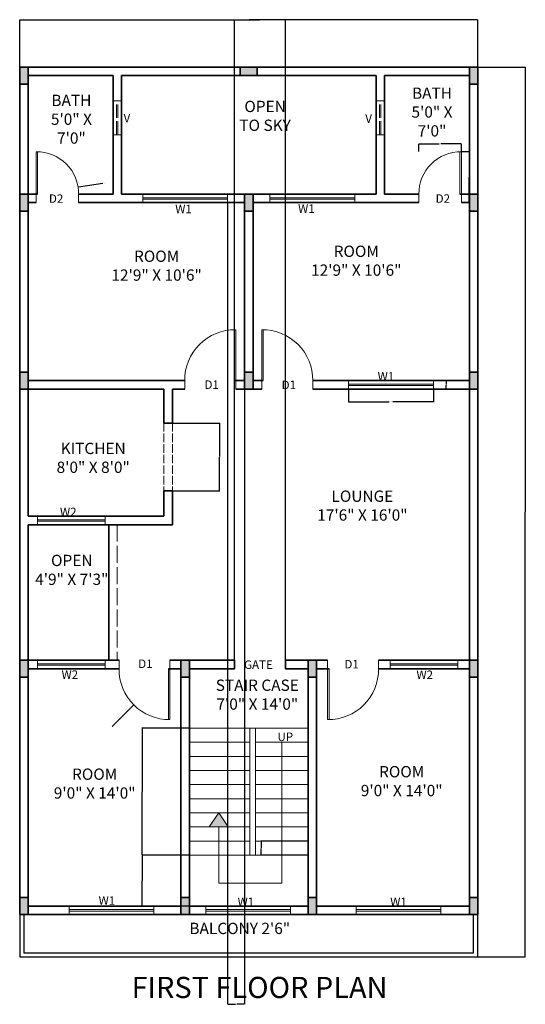
# Model space of a CAD drawing. Units: inches. Extents: x -1239 to -402, y 1021 to 1720.
# Tile 2 of 2: x -760 to -402, y 1022 to 1720. Entities that reach past the tile are written whole.
import ezdxf

# ---------------------------------------------------------------- set-up
doc = ezdxf.new("R2010")
doc.units = ezdxf.units.IN
doc.linetypes.add('ACAD_ISO02W100', pattern=[15, 12, -3])
for name, color, linetype, lineweight in [('A-ANNO-DIMS', 2, 'Continuous', 18), ('A-ANNO-SYMB', 7, 'Continuous', 18), ('A-ANNO-TEXT', 7, 'Continuous', 18), ('A-ANNO-TITL', 7, 'Continuous', 35), ('A-AREA-IDEN', 7, 'Continuous', 18), ('A-COLS', 7, 'Continuous', 35), ('A-DOOR', 3, 'Continuous', 18), ('A-FLOR-BALC', 7, 'Continuous', 25), ('A-FLOR-STRS', 7, 'Continuous', 18), ('A-GLAZ', 4, 'Continuous', 18), ('A-GLAZ-HIDN', 4, 'ACAD_ISO02W100', 13), ('A-WALL', 7, 'Continuous', 35), ('A-WALL-OVHD', 8, 'ACAD_ISO02W100', 18)]:
    doc.layers.add(name, color=color, linetype=linetype, lineweight=lineweight)
doc.styles.get("Standard").update_dxf_attribs({"font": 'arial.ttf'})
doc.dimstyles.get("Standard").update_dxf_attribs({"dimtxt": 0.18, "dimasz": 0.18, "dimexe": 0.18, "dimexo": 0.0625, "dimgap": 0.09, "dimtad": 0, "dimtih": 1, "dimtoh": 1, "dimdec": 4, "dimzin": 0, "dimdsep": 46, "dimtxsty": 'Standard', "dimcen": 0.09, "dimadec": 0, "dimazin": 0, "dimtfac": 1, "dimtdec": 4, "dimtofl": 0, "dimtmove": 0, "dimatfit": 3, "dimfxl": 1, "dimtolj": 1, "dimtzin": 0, "dimarcsym": 0})

# ---------------------------------------------------------------- blocks, each defined once
blk = doc.blocks.new('DOOR-D1-36IN')
for p, q in [((0, 0), (0, 36)), ((1, 0), (1, 36)), ((0, 0), (0, -6)), ((36, 0), (36, -6))]:
    blk.add_line(p, q)
blk.add_arc((0.5, 0.5), 35.5, 359.19307, 90.80693)
blk = doc.blocks.new('DOOR-D2-30IN')
for p, q in [((0, 0), (0, 30)), ((1, 0), (1, 30)), ((0, 0), (0, -6)), ((30, 0), (30, -6))]:
    blk.add_line(p, q)
blk.add_arc((0.5, 0.5), 29.5, 359.02898, 90.97102)
blk = doc.blocks.new('WINDOW-W1-60IN')
for p, q in [((0, 0), (0, -6)), ((60, 0), (60, -6)), ((0, -2.5), (60, -2.5)), ((0, -3.5), (60, -3.5))]:
    blk.add_line(p, q)
blk = doc.blocks.new('WINDOW-W2-48IN')
for p, q in [((0, 0), (0, 6)), ((0, 3.5), (48, 3.5)), ((0, 2.5), (48, 2.5)), ((48, 0), (48, 6))]:
    blk.add_line(p, q)
blk = doc.blocks.new('COLUMN-6X12IN')
h = blk.add_hatch(color=256)
h.dxf.hatch_style = 1
h.paths.add_polyline_path([(6, 12), (0, 12), (0, 0), (6, 0)])
for p, q in [((0, 12), (6, 12)), ((0, 0), (0, 12)), ((6, 12), (6, 0)), ((6, 0), (0, 0))]:
    blk.add_line(p, q)
blk = doc.blocks.new('VENT-SASH-24IN')
at = {"ltscale": 0.8}
for p, q in [((0, 0), (0, -24)), ((1, 0), (1, -24))]:
    blk.add_line(p, q, dxfattribs=at)
blk = doc.blocks.new('*D11')
at = {"layer": 'A-ANNO-DIMS', "color": 0, "lineweight": -2, "transparency": 16777216}
for p, q in [((-447.56, 1626.16), (-442.02, 1626.16)), ((-442.2, 1625.98), (-442.2, 1608.28)), ((-442.2, 1590.21), (-442.2, 1607.91)), ((-447.56, 1590.03), (-442.02, 1590.03))]:
    blk.add_line(p, q, dxfattribs=at)
at = {"layer": 'A-ANNO-DIMS', "color": 0, "transparency": 16777216}
for points in [[(-442.23, 1625.98), (-442.17, 1625.98), (-442.2, 1626.16)], [(-442.23, 1590.21), (-442.17, 1590.21), (-442.2, 1590.03)]]:
    blk.add_solid(points, dxfattribs=at)
at = {"layer": 'Defpoints', "color": 0, "transparency": 16777216}
for p in [(-447.62, 1626.16), (-442.2, 1626.16), (-447.62, 1590.03)]:
    blk.add_point(p, dxfattribs=at)
at = {"layer": 'A-ANNO-DIMS', "color": 0, "transparency": 16777216, "insert": (-442.2, 1608.1), "char_height": 0.18, "attachment_point": 5}
blk.add_mtext('\\A1;DOOR D2 36 TYP.', dxfattribs=at)
blk = doc.blocks.new('*D12')
at = {"layer": 'A-ANNO-DIMS', "color": 0, "lineweight": -2, "transparency": 16777216}
for p, q in [((-477.75, 1626.23), (-477.75, 1631.76)), ((-477.57, 1631.58), (-463.21, 1631.58)), ((-447.8, 1631.58), (-462.16, 1631.58)), ((-447.62, 1626.23), (-447.62, 1631.76))]:
    blk.add_line(p, q, dxfattribs=at)
at = {"layer": 'A-ANNO-DIMS', "color": 0, "transparency": 16777216}
for points in [[(-477.57, 1631.61), (-477.57, 1631.55), (-477.75, 1631.58)], [(-447.8, 1631.61), (-447.8, 1631.55), (-447.62, 1631.58)]]:
    blk.add_solid(points, dxfattribs=at)
at = {"layer": 'Defpoints', "color": 0, "transparency": 16777216}
for p in [(-477.75, 1631.58), (-477.75, 1626.16), (-447.62, 1626.16)]:
    blk.add_point(p, dxfattribs=at)
at = {"layer": 'A-ANNO-DIMS', "color": 0, "transparency": 16777216, "insert": (-462.69, 1631.58), "char_height": 0.18, "attachment_point": 5}
blk.add_mtext('\\A1;30 TYP.', dxfattribs=at)
blk = doc.blocks.new('*D13')
at = {"layer": 'A-ANNO-DIMS', "color": 0, "lineweight": -2, "transparency": 16777216}
for p, q in [((-527.33, 1457.97), (-527.33, 1448.85)), ((-467.33, 1457.97), (-467.33, 1448.85)), ((-527.15, 1449.03), (-498.67, 1449.03)), ((-467.51, 1449.03), (-495.99, 1449.03))]:
    blk.add_line(p, q, dxfattribs=at)
at = {"layer": 'A-ANNO-DIMS', "color": 0, "transparency": 16777216}
for points in [[(-527.15, 1449.06), (-527.15, 1449), (-527.33, 1449.03)], [(-467.51, 1449.06), (-467.51, 1449), (-467.33, 1449.03)]]:
    blk.add_solid(points, dxfattribs=at)
at = {"layer": 'Defpoints', "color": 0, "transparency": 16777216}
for p in [(-527.33, 1458.03), (-467.33, 1458.03), (-467.33, 1449.03)]:
    blk.add_point(p, dxfattribs=at)
at = {"layer": 'A-ANNO-DIMS', "color": 0, "transparency": 16777216, "insert": (-497.33, 1449.03), "char_height": 0.18, "attachment_point": 5}
blk.add_mtext('\\A1;WINDOW W1 60 TYP.', dxfattribs=at)
blk = doc.blocks.new('*D14')
at = {"layer": 'A-ANNO-DIMS', "color": 0, "lineweight": -2, "transparency": 16777216}
for p, q in [((-467.27, 1464.03), (-458.15, 1464.03)), ((-458.33, 1463.85), (-458.33, 1461.21)), ((-467.27, 1458.03), (-458.15, 1458.03)), ((-458.33, 1458.21), (-458.33, 1460.85))]:
    blk.add_line(p, q, dxfattribs=at)
at = {"layer": 'A-ANNO-DIMS', "color": 0, "transparency": 16777216}
for points in [[(-458.36, 1463.85), (-458.3, 1463.85), (-458.33, 1464.03)], [(-458.36, 1458.21), (-458.3, 1458.21), (-458.33, 1458.03)]]:
    blk.add_solid(points, dxfattribs=at)
at = {"layer": 'Defpoints', "color": 0, "transparency": 16777216}
for p in [(-467.33, 1464.03), (-458.33, 1464.03), (-467.33, 1458.03)]:
    blk.add_point(p, dxfattribs=at)
at = {"layer": 'A-ANNO-DIMS', "color": 0, "transparency": 16777216, "insert": (-458.33, 1461.03), "char_height": 0.18, "attachment_point": 5}
blk.add_mtext('\\A1;6 TYP.', dxfattribs=at)
blk = doc.blocks.new('*D21')
at = {"layer": 'A-ANNO-DIMS', "color": 0, "lineweight": -2, "transparency": 16777216}
for p, q in [((-759.96, 1686.09), (-759.96, 1719.56)), ((-759.78, 1719.38), (-598.25, 1719.38)), ((-436.14, 1719.38), (-597.68, 1719.38)), ((-435.96, 1686.09), (-435.96, 1719.56))]:
    blk.add_line(p, q, dxfattribs=at)
at = {"layer": 'A-ANNO-DIMS', "color": 0, "transparency": 16777216}
for points in [[(-759.78, 1719.41), (-759.78, 1719.35), (-759.96, 1719.38)], [(-436.14, 1719.41), (-436.14, 1719.35), (-435.96, 1719.38)]]:
    blk.add_solid(points, dxfattribs=at)
at = {"layer": 'Defpoints', "color": 0, "transparency": 16777216}
for p in [(-435.96, 1719.38), (-759.96, 1686.03), (-435.96, 1686.03)]:
    blk.add_point(p, dxfattribs=at)
at = {"layer": 'A-ANNO-DIMS', "color": 0, "transparency": 16777216, "insert": (-597.96, 1719.38), "char_height": 0.18, "attachment_point": 5}
blk.add_mtext('\\A1;324', dxfattribs=at)
blk = doc.blocks.new('*D22')
at = {"layer": 'A-ANNO-DIMS', "color": 0, "lineweight": -2, "transparency": 16777216}
for p, q in [((-435.9, 1686.03), (-402.43, 1686.03)), ((-402.61, 1685.85), (-402.61, 1371.21)), ((-402.61, 1056.21), (-402.61, 1370.85)), ((-435.9, 1056.03), (-402.43, 1056.03))]:
    blk.add_line(p, q, dxfattribs=at)
at = {"layer": 'A-ANNO-DIMS', "color": 0, "transparency": 16777216}
for points in [[(-402.64, 1685.85), (-402.58, 1685.85), (-402.61, 1686.03)], [(-402.64, 1056.21), (-402.58, 1056.21), (-402.61, 1056.03)]]:
    blk.add_solid(points, dxfattribs=at)
at = {"layer": 'Defpoints', "color": 0, "transparency": 16777216}
for p in [(-435.96, 1686.03), (-402.61, 1686.03), (-435.96, 1056.03)]:
    blk.add_point(p, dxfattribs=at)
at = {"layer": 'A-ANNO-DIMS', "color": 0, "transparency": 16777216, "insert": (-402.61, 1371.03), "char_height": 0.18, "attachment_point": 5}
blk.add_mtext('\\A1;630', dxfattribs=at)
blk = doc.blocks.new('*D31')
at = {"layer": 'A-ANNO-DIMS', "color": 0, "lineweight": -2, "transparency": 16777216}
for p, q in [((-640.03, 1218.03), (-673.49, 1218.03)), ((-673.31, 1217.85), (-673.31, 1173.21)), ((-673.31, 1128.21), (-673.31, 1172.85)), ((-640.03, 1128.03), (-673.49, 1128.03))]:
    blk.add_line(p, q, dxfattribs=at)
at = {"layer": 'A-ANNO-DIMS', "color": 0, "transparency": 16777216}
for points in [[(-673.34, 1217.85), (-673.28, 1217.85), (-673.31, 1218.03)], [(-673.34, 1128.21), (-673.28, 1128.21), (-673.31, 1128.03)]]:
    blk.add_solid(points, dxfattribs=at)
at = {"layer": 'Defpoints', "color": 0, "transparency": 16777216}
for p in [(-673.31, 1218.03), (-639.96, 1218.03), (-639.96, 1128.03)]:
    blk.add_point(p, dxfattribs=at)
at = {"layer": 'A-ANNO-DIMS', "color": 0, "transparency": 16777216, "insert": (-673.31, 1173.03), "char_height": 0.18, "attachment_point": 5}
blk.add_mtext('\\A1;90', dxfattribs=at)
blk = doc.blocks.new('*D32')
at = {"layer": 'A-ANNO-DIMS', "color": 0, "lineweight": -2, "transparency": 16777216}
for p, q in [((-556.03, 1138.03), (-589.49, 1138.03)), ((-589.31, 1137.85), (-589.31, 1133.21)), ((-589.31, 1128.21), (-589.31, 1132.85)), ((-556.03, 1128.03), (-589.49, 1128.03))]:
    blk.add_line(p, q, dxfattribs=at)
at = {"layer": 'A-ANNO-DIMS', "color": 0, "transparency": 16777216}
for points in [[(-589.34, 1137.85), (-589.28, 1137.85), (-589.31, 1138.03)], [(-589.34, 1128.21), (-589.28, 1128.21), (-589.31, 1128.03)]]:
    blk.add_solid(points, dxfattribs=at)
at = {"layer": 'Defpoints', "color": 0, "transparency": 16777216}
for p in [(-589.31, 1138.03), (-555.96, 1138.03), (-555.96, 1128.03)]:
    blk.add_point(p, dxfattribs=at)
at = {"layer": 'A-ANNO-DIMS', "color": 0, "transparency": 16777216, "insert": (-589.31, 1133.03), "char_height": 0.18, "attachment_point": 5}
blk.add_mtext('\\A1;10', dxfattribs=at)
blk = doc.blocks.new('*D33')
at = {"layer": 'A-ANNO-DIMS', "color": 0, "lineweight": -2, "transparency": 16777216}
for p, q in [((-640.03, 1128.03), (-673.49, 1128.03)), ((-673.31, 1127.85), (-673.31, 1110.21)), ((-673.31, 1092.21), (-673.31, 1109.85)), ((-640.03, 1092.03), (-673.49, 1092.03))]:
    blk.add_line(p, q, dxfattribs=at)
at = {"layer": 'A-ANNO-DIMS', "color": 0, "transparency": 16777216}
for points in [[(-673.34, 1127.85), (-673.28, 1127.85), (-673.31, 1128.03)], [(-673.34, 1092.21), (-673.28, 1092.21), (-673.31, 1092.03)]]:
    blk.add_solid(points, dxfattribs=at)
at = {"layer": 'Defpoints', "color": 0, "transparency": 16777216}
for p in [(-673.31, 1128.03), (-639.96, 1128.03), (-639.96, 1092.03)]:
    blk.add_point(p, dxfattribs=at)
at = {"layer": 'A-ANNO-DIMS', "color": 0, "transparency": 16777216, "insert": (-673.31, 1110.03), "char_height": 0.18, "attachment_point": 5}
blk.add_mtext('\\A1;36', dxfattribs=at)
blk = doc.blocks.new('*D34')
at = {"layer": 'A-ANNO-DIMS', "color": 0, "lineweight": -2, "transparency": 16777216}
for p, q in [((-608.1, 1266.09), (-608.1, 1719.56)), ((-607.92, 1719.38), (-590.32, 1719.38)), ((-572.28, 1719.38), (-589.88, 1719.38)), ((-572.1, 1266.09), (-572.1, 1719.56))]:
    blk.add_line(p, q, dxfattribs=at)
at = {"layer": 'A-ANNO-DIMS', "color": 0, "transparency": 16777216}
for points in [[(-607.92, 1719.41), (-607.92, 1719.35), (-608.1, 1719.38)], [(-572.28, 1719.41), (-572.28, 1719.35), (-572.1, 1719.38)]]:
    blk.add_solid(points, dxfattribs=at)
at = {"layer": 'Defpoints', "color": 0, "transparency": 16777216}
for p in [(-572.1, 1719.38), (-608.1, 1266.03), (-572.1, 1266.03)]:
    blk.add_point(p, dxfattribs=at)
at = {"layer": 'A-ANNO-DIMS', "color": 0, "transparency": 16777216, "insert": (-590.1, 1719.38), "char_height": 0.18, "attachment_point": 5}
blk.add_mtext('\\A1;36', dxfattribs=at)
blk = doc.blocks.new('*D35')
at = {"layer": 'A-ANNO-DIMS', "color": 0, "lineweight": -2, "transparency": 16777216}
for p, q in [((-651.9, 1434.03), (-618.43, 1434.03)), ((-618.61, 1433.85), (-618.61, 1410.21)), ((-618.61, 1386.21), (-618.61, 1409.85)), ((-651.9, 1386.03), (-618.43, 1386.03))]:
    blk.add_line(p, q, dxfattribs=at)
at = {"layer": 'A-ANNO-DIMS', "color": 0, "transparency": 16777216}
for points in [[(-618.64, 1433.85), (-618.58, 1433.85), (-618.61, 1434.03)], [(-618.64, 1386.21), (-618.58, 1386.21), (-618.61, 1386.03)]]:
    blk.add_solid(points, dxfattribs=at)
at = {"layer": 'Defpoints', "color": 0, "transparency": 16777216}
for p in [(-651.96, 1434.03), (-651.96, 1386.03), (-618.61, 1386.03)]:
    blk.add_point(p, dxfattribs=at)
at = {"layer": 'A-ANNO-DIMS', "color": 0, "transparency": 16777216, "insert": (-618.61, 1410.03), "char_height": 0.18, "attachment_point": 5}
blk.add_mtext('\\A1;48', dxfattribs=at)
blk = doc.blocks.new('*D37')
at = {"layer": 'A-ANNO-DIMS', "color": 0, "lineweight": -2, "transparency": 16777216}
for p, q in [((-612.96, 1589.97), (-612.96, 1022.5)), ((-600.96, 1589.97), (-600.96, 1022.5)), ((-612.78, 1022.68), (-607.42, 1022.68)), ((-601.14, 1022.68), (-606.51, 1022.68))]:
    blk.add_line(p, q, dxfattribs=at)
at = {"layer": 'A-ANNO-DIMS', "color": 0, "transparency": 16777216}
for points in [[(-612.78, 1022.71), (-612.78, 1022.65), (-612.96, 1022.68)], [(-601.14, 1022.71), (-601.14, 1022.65), (-600.96, 1022.68)]]:
    blk.add_solid(points, dxfattribs=at)
at = {"layer": 'Defpoints', "color": 0, "transparency": 16777216}
for p in [(-612.96, 1590.03), (-600.96, 1590.03), (-600.96, 1022.68)]:
    blk.add_point(p, dxfattribs=at)
at = {"layer": 'A-ANNO-DIMS', "color": 0, "transparency": 16777216, "insert": (-606.96, 1022.68), "char_height": 0.18, "attachment_point": 5}
blk.add_mtext('\\A1;11.998', dxfattribs=at)
blk = doc.blocks.new('*D41')
at = {"layer": 'A-ANNO-DIMS', "color": 0, "lineweight": -2, "transparency": 16777216}
for p, q in [((-654.32, 1259.53), (-654.14, 1259.53)), ((-654.23, 1259.44), (-654.23, 1259.62)), ((-694.39, 1219.36), (-679.46, 1234.3)), ((-694.57, 1219.36), (-694.39, 1219.36))]:
    blk.add_line(p, q, dxfattribs=at)
at = {"layer": 'A-ANNO-DIMS', "color": 0, "transparency": 16777216}
blk.add_solid([(-679.48, 1234.32), (-679.44, 1234.27), (-679.33, 1234.42)], dxfattribs=at)
at = {"layer": 'Defpoints', "color": 0, "transparency": 16777216}
for p in [(-654.23, 1259.53), (-679.33, 1234.42)]:
    blk.add_point(p, dxfattribs=at)
at = {"layer": 'A-ANNO-DIMS', "color": 0, "transparency": 16777216, "insert": (-695.18, 1219.36), "char_height": 0.18, "attachment_point": 5}
blk.add_mtext('\\A1;4X R35.5', dxfattribs=at)
blk = doc.blocks.new('*D42')
at = {"layer": 'A-ANNO-DIMS', "color": 0, "lineweight": -2, "transparency": 16777216}
for p, q in [((-701.13, 1603.53), (-718.45, 1600.93)), ((-747.9, 1596.53), (-747.72, 1596.53)), ((-747.81, 1596.44), (-747.81, 1596.62))]:
    blk.add_line(p, q, dxfattribs=at)
at = {"layer": 'A-ANNO-DIMS', "color": 0, "transparency": 16777216}
blk.add_solid([(-718.46, 1600.96), (-718.45, 1600.9), (-718.63, 1600.91)], dxfattribs=at)
at = {"layer": 'Defpoints', "color": 0, "transparency": 16777216}
for p in [(-747.81, 1596.53), (-718.63, 1600.91)]:
    blk.add_point(p, dxfattribs=at)
at = {"layer": 'A-ANNO-DIMS', "color": 0, "transparency": 16777216, "insert": (-700.38, 1603.53), "char_height": 0.18, "attachment_point": 5}
blk.add_mtext('\\A1;2X R29.504', dxfattribs=at)

msp = doc.modelspace()

# ---------------------------------------------------------------- hatches: boundary and pattern name
at = {"layer": 'A-ANNO-SYMB'}
h = msp.add_hatch(color=256, dxfattribs=at)
h.dxf.hatch_style = 1
h.paths.add_polyline_path([(-612.5246, 1148.028), (-619.2064, 1158.028), (-625.8883, 1148.028)])

# ---------------------------------------------------------------- linework, layer by layer
for p, q in [((-574.56, 1208.028), (-574.56, 1108.2999)), ((-619.2064, 1158.028), (-625.8883, 1148.028)), ((-619.2064, 1158.028), (-612.5246, 1148.028)), ((-619.2064, 1108.2999), (-619.2064, 1148.028)), ((-574.56, 1108.2999), (-619.2064, 1108.2999))]:
    msp.add_line(p, q, dxfattribs=at)
at = {"layer": 'A-FLOR-BALC'}
for p, q in [((-759.9646, 1086.028), (-759.9646, 1056.028)), ((-756.9646, 1086.028), (-756.9646, 1059.028)), ((-438.9646, 1059.028), (-438.9646, 1086.028)), ((-435.9646, 1056.028), (-435.9646, 1086.028)), ((-759.9646, 1056.028), (-435.9646, 1056.028)), ((-756.9646, 1059.028), (-438.9646, 1059.028))]:
    msp.add_line(p, q, dxfattribs=at)
at = {"layer": 'A-FLOR-STRS'}
for p, q in [((-639.9646, 1218.028), (-597.1554, 1218.028)), ((-597.1554, 1218.028), (-555.9646, 1218.028)), ((-597.1554, 1128.028), (-597.1554, 1218.028)), ((-593.1554, 1128.028), (-593.1554, 1218.028)), ((-639.9646, 1208.028), (-597.1554, 1208.028)), ((-593.1554, 1208.028), (-555.9646, 1208.028)), ((-639.9646, 1198.028), (-597.1554, 1198.028)), ((-593.1554, 1198.028), (-555.9646, 1198.028)), ((-639.9646, 1188.028), (-597.1554, 1188.028)), ((-593.1554, 1188.028), (-555.9646, 1188.028)), ((-639.9646, 1178.028), (-597.1554, 1178.028)), ((-593.1554, 1178.028), (-555.9646, 1178.028)), ((-639.9646, 1168.028), (-597.1554, 1168.028)), ((-593.1554, 1168.028), (-555.9646, 1168.028)), ((-639.9646, 1158.028), (-597.1554, 1158.028)), ((-593.1554, 1158.028), (-555.9646, 1158.028)), ((-639.9646, 1148.028), (-597.1554, 1148.028)), ((-593.1554, 1148.028), (-555.9646, 1148.028)), ((-639.9646, 1138.028), (-597.1554, 1138.028)), ((-593.1554, 1138.028), (-555.9646, 1138.028)), ((-639.9646, 1128.028), (-597.1554, 1128.028)), ((-597.1554, 1128.028), (-555.9646, 1128.028))]:
    msp.add_line(p, q, dxfattribs=at)
at = {"layer": 'A-GLAZ'}
for p, q in [((-693.9646, 1662.028), (-687.9646, 1662.028)), ((-507.9646, 1662.028), (-501.9646, 1662.028)), ((-693.9646, 1638.028), (-687.9646, 1638.028)), ((-507.9646, 1638.028), (-501.9646, 1638.028))]:
    msp.add_line(p, q, dxfattribs=at)
at = {"layer": 'A-WALL'}
for p, q in [((-435.9646, 1686.028), (-759.9646, 1686.028)), ((-759.9646, 1686.028), (-759.9646, 1086.028)), ((-693.9646, 1680.028), (-753.9646, 1680.028)), ((-753.9646, 1680.028), (-753.9646, 1596.028)), ((-693.9646, 1680.028), (-693.9646, 1596.028)), ((-507.9646, 1680.028), (-687.9646, 1680.028)), ((-687.9646, 1680.028), (-687.9646, 1596.028)), ((-507.9646, 1596.028), (-507.9646, 1680.028)), ((-441.9646, 1680.028), (-501.9646, 1680.028)), ((-501.9646, 1596.028), (-501.9646, 1680.028)), ((-441.9646, 1596.028), (-441.9646, 1680.028)), ((-435.9646, 1086.028), (-435.9646, 1686.028)), ((-753.9646, 1596.028), (-747.31, 1596.028)), ((-753.9646, 1590.028), (-753.9646, 1464.028)), ((-753.9646, 1590.028), (-748.31, 1590.028)), ((-718.31, 1596.028), (-693.9646, 1596.028)), ((-718.31, 1590.028), (-600.9646, 1590.028)), ((-687.9646, 1596.028), (-507.9646, 1596.028)), ((-600.9646, 1590.028), (-600.9646, 1464.028)), ((-594.9646, 1590.028), (-477.6192, 1590.028)), ((-594.9646, 1464.028), (-594.9646, 1590.028)), ((-501.9646, 1596.028), (-477.6192, 1596.028)), ((-448.6192, 1596.028), (-441.9646, 1596.028)), ((-447.6192, 1590.028), (-441.9646, 1590.028)), ((-441.9646, 1464.028), (-441.9646, 1590.028)), ((-753.9646, 1464.028), (-643.2306, 1464.028)), ((-608.2306, 1464.028), (-600.9646, 1464.028)), ((-594.9646, 1464.028), (-587.6985, 1464.028)), ((-552.6985, 1464.028), (-441.9646, 1464.028)), ((-753.9646, 1458.028), (-753.9646, 1368.028)), ((-753.9646, 1458.028), (-657.9646, 1458.028)), ((-657.9646, 1458.028), (-657.9646, 1434.028)), ((-651.9646, 1458.028), (-651.9646, 1434.028)), ((-651.9646, 1458.028), (-643.2306, 1458.028)), ((-607.2306, 1458.028), (-588.6985, 1458.028)), ((-552.6985, 1458.028), (-441.9646, 1458.028)), ((-441.9646, 1266.028), (-441.9646, 1458.028)), ((-651.9646, 1434.028), (-657.9646, 1434.028)), ((-657.9646, 1386.028), (-657.9646, 1368.028)), ((-651.9646, 1386.028), (-657.9646, 1386.028)), ((-651.9646, 1386.028), (-651.9646, 1362.028)), ((-753.9646, 1368.028), (-657.9646, 1368.028)), ((-753.9646, 1362.028), (-753.9646, 1266.028)), ((-753.9646, 1362.028), (-651.9646, 1362.028)), ((-696.9646, 1362.028), (-696.9646, 1266.028)), ((-753.9646, 1266.028), (-689.7251, 1266.028)), ((-653.7251, 1266.028), (-608.0997, 1266.028)), ((-608.0997, 1266.028), (-608.0997, 1260.028)), ((-572.0997, 1266.028), (-542.204, 1266.028)), ((-572.0997, 1266.028), (-572.0997, 1260.028)), ((-506.204, 1266.028), (-441.9646, 1266.028)), ((-753.9646, 1260.028), (-753.9646, 1092.028)), ((-753.9646, 1260.028), (-689.7251, 1260.028)), ((-654.7251, 1260.028), (-645.9646, 1260.028)), ((-645.9646, 1260.028), (-645.9646, 1092.028)), ((-639.9646, 1260.028), (-639.9646, 1092.028)), ((-639.9646, 1260.028), (-608.0997, 1260.028)), ((-572.0997, 1260.028), (-555.9646, 1260.028)), ((-555.9646, 1092.028), (-555.9646, 1260.028)), ((-549.9646, 1260.028), (-541.204, 1260.028)), ((-549.9646, 1092.028), (-549.9646, 1260.028)), ((-506.204, 1260.028), (-441.9646, 1260.028)), ((-441.9646, 1092.028), (-441.9646, 1260.028)), ((-753.9646, 1092.028), (-744.2122, 1092.028)), ((-744.2122, 1092.028), (-645.9646, 1092.028)), ((-639.9646, 1092.028), (-592.3462, 1092.028)), ((-592.3462, 1092.028), (-555.9646, 1092.028)), ((-549.9646, 1092.028), (-541.204, 1092.028)), ((-542.204, 1092.028), (-441.9646, 1092.028)), ((-759.9646, 1086.028), (-744.2122, 1086.028)), ((-744.2122, 1086.028), (-592.3462, 1086.028)), ((-592.3462, 1086.028), (-542.204, 1086.028)), ((-542.204, 1086.028), (-435.9646, 1086.028))]:
    msp.add_line(p, q, dxfattribs=at)
at = {"layer": 'A-WALL-OVHD', "ltscale": 0.5}
for p, q in [((-657.9646, 1434.028), (-657.9646, 1386.028)), ((-651.9646, 1434.028), (-651.9646, 1386.028))]:
    msp.add_line(p, q, dxfattribs=at)
at = {"layer": 'A-WALL-OVHD'}
msp.add_line((-690.9646, 1362.028), (-690.9646, 1266.028), dxfattribs=at)

# ---------------------------------------------------------------- block references
at = {"layer": 'A-COLS'}
for p in [(-759.9646, 1674.028), (-441.9646, 1674.028), (-759.9646, 1584.028), (-600.9646, 1584.028), (-441.9646, 1584.028), (-759.9646, 1458.028), (-600.9646, 1458.028), (-441.9646, 1458.028), (-759.9646, 1254.028), (-645.9646, 1254.028), (-555.9646, 1254.028), (-441.9646, 1254.028), (-759.9646, 1086.028), (-645.9646, 1086.028), (-555.9646, 1086.028), (-441.9646, 1086.028)]:
    msp.add_blockref('COLUMN-6X12IN', p, dxfattribs=at)
at = {"layer": 'A-COLS', "rotation": 89.999999999998}
msp.add_blockref('COLUMN-6X12IN', (-591.9646, 1680.028), dxfattribs=at)
at = {"layer": 'A-DOOR'}
for name, p in [('DOOR-D2-30IN', (-748.31, 1596.028)), ('DOOR-D1-36IN', (-588.6985, 1464.028))]:
    msp.add_blockref(name, p, dxfattribs=at)
at = {"layer": 'A-DOOR', "extrusion": (0, 0, -1), "zscale": -1}
for name, p in [('DOOR-D2-30IN', (447.6192, 1596.028)), ('DOOR-D1-36IN', (607.2306, 1464.028))]:
    msp.add_blockref(name, p, dxfattribs=at)
at = {"layer": 'A-DOOR', "rotation": 180}
msp.add_blockref('DOOR-D1-36IN', (-653.7251, 1260.028), dxfattribs=at)
at = {"layer": 'A-DOOR', "extrusion": (0, 0, -1), "zscale": -1, "rotation": 180}
msp.add_blockref('DOOR-D1-36IN', (542.204, 1260.028), dxfattribs=at)
at = {"layer": 'A-GLAZ'}
for name, p in [('WINDOW-W1-60IN', (-672.9624, 1596.028)), ('WINDOW-W1-60IN', (-527.3315, 1464.028)), ('WINDOW-W2-48IN', (-498.0843, 1260.028))]:
    msp.add_blockref(name, p, dxfattribs=at)
at = {"layer": 'A-GLAZ', "rotation": 180}
for name, p in [('WINDOW-W1-60IN', (-522.9668, 1590.028)), ('WINDOW-W2-48IN', (-699.4305, 1368.028)), ('WINDOW-W2-48IN', (-699.4305, 1266.028)), ('WINDOW-W1-60IN', (-665.0884, 1086.028)), ('WINDOW-W1-60IN', (-568.4286, 1086.028)), ('WINDOW-W1-60IN', (-462.0843, 1086.028))]:
    msp.add_blockref(name, p, dxfattribs=at)
at = {"layer": 'A-GLAZ-HIDN', "rotation": 180}
for p in [(-690.4646, 1638.028), (-504.4646, 1638.028)]:
    msp.add_blockref('VENT-SASH-24IN', p, dxfattribs=at)

# ---------------------------------------------------------------- texts
at = {"layer": 'A-ANNO-TEXT', "char_height": 6, "attachment_point": 1}
for s, width, insert in [('V', 21.819943, (-686.493, 1652.8943)), ('V', 21.819943, (-515.5796, 1652.5221)), ('D2', 21.819943, (-739.2931, 1595.9048)), ('D2', 21.819943, (-465.8001, 1595.933)), ('W1', 21.819943, (-649.9534, 1588.5129)), ('W1', 21.819943, (-563.0907, 1588.7928)), ('D1', 21.819943, (-629.2758, 1464.1788)), ('D1', 21.819943, (-574.7319, 1464.0085)), ('W1', 21.819943, (-506.8286, 1470.0526)), ('W2', 21.819943, (-731.491, 1374.0526)), ('D1', 21.819943, (-676.1475, 1266.5784)), ('GATE', 57.104456, (-601.2869, 1265.9537)), ('D1', 21.819943, (-530.3115, 1266.2834)), ('W2', 21.819943, (-730.3917, 1258.8998)), ('W2', 21.819943, (-479.3815, 1258.7733)), ('UP', 21.819943, (-577.6561, 1214.8762)), ('W1', 21.819943, (-704.1706, 1098.9555)), ('W1', 21.819943, (-605.8696, 1098.0526)), ('W1', 21.819943, (-497.9079, 1098.0526))]:
    msp.add_mtext_dynamic_manual_height_columns(s, width=width, gutter_width=12.5, heights=[0], dxfattribs=dict(at, insert=insert))
at = {"layer": 'A-ANNO-TITL', "insert": (-734.5624, 1041.9277), "char_height": 15, "attachment_point": 1}
msp.add_mtext_dynamic_manual_height_columns('\\pxqc;{\\fArial|b1|i0|c0|p34;FIRST FLOOR PLAN}', width=288.409032, gutter_width=12.5, heights=[0], dxfattribs=at)
at = {"layer": 'A-AREA-IDEN', "char_height": 8, "attachment_point": 1}
for s, width, insert in [('\\pxqc;BATH\\P5\'0" X 7\'0"', 50.533842, (-748.6682, 1666.432)), ('\\pxqc;BATH\\P5\'0" X 7\'0"', 50.533842, (-493.6383, 1671.5305)), ('\\pxqc;OPEN\\PTO SKY', 61.660387, (-617.2553, 1662.1456)), ('\\pxqc;ROOM\\P12\'9" X 10\'6"', 86.734176, (-706.5093, 1556.0826)), ('\\pxqc;ROOM\\P12\'9" X 10\'6"', 86.734176, (-565.3012, 1559.5899)), ('\\pxqc;KITCHEN\\P8\'0" X 8\'0"', 86.734176, (-751.3627, 1420.0287)), ('\\pxqc;LOUNGE\\P17\'6" X 16\'0"', 86.734176, (-560.9783, 1386.2223)), ('\\pxqc;OPEN\\P4\'9" X 7\'3"', 61.660387, (-753.9646, 1340.7271)), ('\\pxqc;STAIR CASE\\P7\'0" X 14\'0"', 86.734176, (-635.3001, 1252.3765)), ('\\pxqc;ROOM\\P9\'0" X 14\'0"', 86.734176, (-750.3194, 1189.4315)), ('\\pxqc;ROOM\\P9\'0" X 14\'0"', 86.734176, (-533.1853, 1191.1766)), ('\\pxqc;BALCONY 2\'6"', 86.625162, (-647.6521, 1080.2306))]:
    msp.add_mtext_dynamic_manual_height_columns(s, width=width, gutter_width=12.5, heights=[0], dxfattribs=dict(at, insert=insert))

# ---------------------------------------------------------------- dimensions: what is measured, and where the dimension line sits
at = {"layer": 'A-ANNO-DIMS'}
for base, p1, p2, override, picture, middle in [((-435.9646, 1719.378), (-759.9646, 1686.028), (-435.9646, 1686.028), {"dimdec": 0, "dimlfac": 1, "dimrnd": 0, "dimzin": 0, "dimdsep": 46, "dimlunit": 2}, '*D21', (-597.9646, 1719.378)), ((-572.0997, 1719.378), (-608.0997, 1266.028), (-572.0997, 1266.028), {"dimdec": 0, "dimlfac": 1, "dimrnd": 0, "dimzin": 0, "dimdsep": 46, "dimlunit": 2}, '*D34', (-590.0997, 1719.378)), ((-600.9646, 1022.678), (-612.9624, 1590.028), (-600.9646, 1590.028), {"dimdec": 3, "dimlfac": 1, "dimrnd": 0, "dimzin": 0, "dimdsep": 46, "dimlunit": 2}, '*D37', (-606.9635, 1022.678))]:
    dim = msp.add_linear_dim(base=base, p1=p1, p2=p2, dimstyle='Standard', override=override, dxfattribs=at)
    dim.commit()
    dim.dimension.update_dxf_attribs({"geometry": picture, "text_midpoint": middle})
for base, p1, p2, angle, picture, middle in [((-402.6146, 1686.028), (-435.9646, 1056.028), (-435.9646, 1686.028), 90, '*D22', (-402.6146, 1371.028)), ((-618.6146, 1386.028), (-651.9646, 1434.028), (-651.9646, 1386.028), 270, '*D35', (-618.6146, 1410.028)), ((-673.3146, 1218.028), (-639.9646, 1128.028), (-639.9646, 1218.028), 90, '*D31', (-673.3146, 1173.028)), ((-589.3146, 1138.028), (-555.9646, 1128.028), (-555.9646, 1138.028), 90, '*D32', (-589.3146, 1133.028)), ((-673.3146, 1128.028), (-639.9646, 1092.028), (-639.9646, 1128.028), 90, '*D33', (-673.3146, 1110.028))]:
    dim = msp.add_linear_dim(base=base, p1=p1, p2=p2, angle=angle, dimstyle='Standard', override={"dimdec": 0, "dimlfac": 1, "dimrnd": 0, "dimzin": 0, "dimdsep": 46, "dimlunit": 2}, dxfattribs=at)
    dim.commit()
    dim.dimension.update_dxf_attribs({"geometry": picture, "text_midpoint": middle})
for base, p1, p2, angle, text, picture, middle in [((-477.7547, 1631.5839), (-447.6192, 1626.1636), (-477.7547, 1626.1636), 180, '<> TYP.', '*D12', (-462.6869, 1631.5839)), ((-442.1988, 1626.1636), (-447.6192, 1590.028), (-447.6192, 1626.1636), 90, 'DOOR D2 <> TYP.', '*D11', (-442.1988, 1608.0958)), ((-458.3315, 1464.028), (-467.3315, 1458.028), (-467.3315, 1464.028), 90, '<> TYP.', '*D14', (-458.3315, 1461.028))]:
    dim = msp.add_linear_dim(base=base, p1=p1, p2=p2, angle=angle, text=text, dimstyle='Standard', override={"dimdec": 0, "dimlfac": 1, "dimrnd": 0, "dimzin": 0, "dimdsep": 46, "dimlunit": 2}, dxfattribs=at)
    dim.commit()
    dim.dimension.update_dxf_attribs({"geometry": picture, "text_midpoint": middle})
for center, mpoint, text, override, picture, middle in [((-747.81, 1596.528), (-718.6324, 1600.9062), '2X <>', {"dimdec": 3, "dimlfac": 1, "dimrnd": 0, "dimzin": 0, "dimdsep": 46, "dimlunit": 2}, '*D42', (-701.1258, 1603.5331)), ((-654.2251, 1259.528), (-679.3298, 1234.4232), '4X <>', {"dimdec": 1, "dimlfac": 1, "dimrnd": 0, "dimzin": 0, "dimdsep": 46, "dimlunit": 2}, '*D41', (-695.1802, 1219.3603))]:
    dim = msp.add_radius_dim(center=center, mpoint=mpoint, text=text, dimstyle='Standard', override=override, dxfattribs=at)
    dim.commit()
    dim.dimension.update_dxf_attribs({"geometry": picture, "text_midpoint": middle, "dimtype": 164})
dim = msp.add_linear_dim(base=(-467.3315, 1449.028), p1=(-527.3315, 1458.028), p2=(-467.3315, 1458.028), text='WINDOW W1 <> TYP.', dimstyle='Standard', override={"dimdec": 0, "dimlfac": 1, "dimrnd": 0, "dimzin": 0, "dimdsep": 46, "dimlunit": 2}, dxfattribs=at)
dim.commit()
dim.dimension.update_dxf_attribs({"geometry": '*D13', "text_midpoint": (-497.3315, 1449.028)})

doc.saveas('drawing.dxf')
